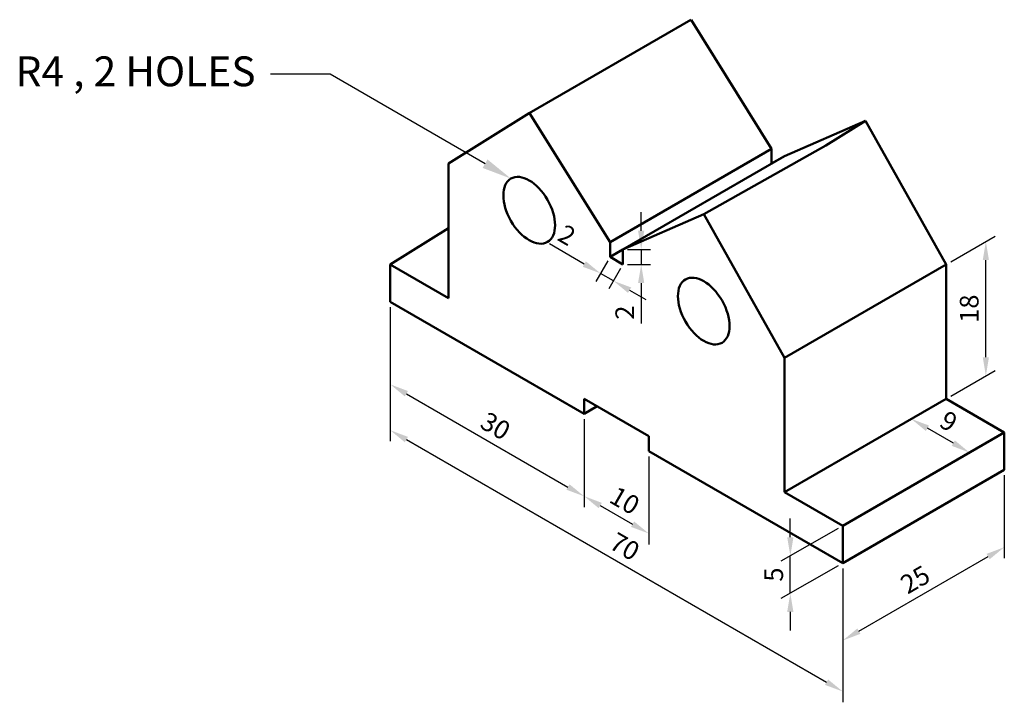
# Model space of a CAD drawing. Units: millimetres. Extents: x 4633 to 4764, y 591 to 682.
import ezdxf
from ezdxf import colors
from ezdxf.entities.mleader import LeaderData, LeaderLine
from ezdxf.math import Vec2, Vec3

# ---------------------------------------------------------------- set-up
doc = ezdxf.new("R2010")
doc.units = ezdxf.units.MM
for name, color, linetype, lineweight in [('M-DIMS', 2, 'Continuous', 25), ('M-OUTL', 7, 'Continuous', 50), ('M-TEXT', 3, 'Continuous', 25)]:
    doc.layers.add(name, color=color, linetype=linetype, lineweight=lineweight)
doc.styles.get("Standard").update_dxf_attribs({"font": 'arial.ttf'})
doc.dimstyles.new('ISO-25', dxfattribs={"dimtxt": 2.5, "dimasz": 2.5, "dimexe": 1.25, "dimexo": 0.625, "dimtad": 1, "dimtxsty": 'Standard', "dimcen": 2.5, "dimadec": 0, "dimazin": 0, "dimtfac": 1, "dimtmove": 0, "dimatfit": 3, "dimfxl": 1, "dimarcsym": 0})

# ---------------------------------------------------------------- blocks, each defined once
blk = doc.blocks.new('*D1')
at = {"layer": 'Defpoints', "color": 0, "transparency": 16777216}
for p in [(4682.17, 644.63), (4708.15, 629.63), (4708.15, 618.56)]:
    blk.add_point(p, dxfattribs=at)
at = {"layer": 'M-DIMS', "color": 0, "lineweight": -2, "transparency": 16777216}
for p, q in [((4682.17, 643.91), (4682.17, 632.12)), ((4684.33, 632.31), (4705.98, 619.81)), ((4708.15, 628.91), (4708.15, 617.12))]:
    blk.add_line(p, q, dxfattribs=at)
at = {"layer": 'M-DIMS', "color": 0, "transparency": 16777216}
for points in [[(4684.54, 632.67), (4684.12, 631.95), (4682.17, 633.56)], [(4706.19, 620.17), (4705.77, 619.45), (4708.15, 618.56)]]:
    blk.add_solid(points, dxfattribs=at)
at = {"layer": 'M-DIMS', "color": 0, "transparency": 16777216, "insert": (4696.11, 627.71), "char_height": 2.5, "attachment_point": 5, "rotation": 330}
blk.add_mtext('30', dxfattribs=at)
blk = doc.blocks.new('*D2')
at = {"layer": 'Defpoints', "color": 0, "transparency": 16777216}
for p in [(4708.15, 629.63), (4716.81, 624.63), (4716.81, 613.58)]:
    blk.add_point(p, dxfattribs=at)
at = {"layer": 'M-DIMS', "color": 0, "lineweight": -2, "transparency": 16777216}
for p, q in [((4708.15, 628.91), (4708.15, 617.13)), ((4716.81, 623.91), (4716.81, 612.13)), ((4710.31, 617.33), (4714.64, 614.83))]:
    blk.add_line(p, q, dxfattribs=at)
at = {"layer": 'M-DIMS', "color": 0, "transparency": 16777216}
for points in [[(4710.52, 617.69), (4710.1, 616.97), (4708.15, 618.58)], [(4714.85, 615.19), (4714.43, 614.47), (4716.81, 613.58)]]:
    blk.add_solid(points, dxfattribs=at)
at = {"layer": 'M-DIMS', "color": 0, "transparency": 16777216, "insert": (4713.43, 617.72), "char_height": 2.5, "attachment_point": 5, "rotation": 330}
blk.add_mtext('10', dxfattribs=at)
blk = doc.blocks.new('*D3')
at = {"layer": 'Defpoints', "color": 0, "transparency": 16777216}
for p in [(4682.17, 644.63), (4742.79, 609.63), (4742.79, 592.42)]:
    blk.add_point(p, dxfattribs=at)
at = {"layer": 'M-DIMS', "color": 0, "lineweight": -2, "transparency": 16777216}
for p, q in [((4682.17, 643.91), (4682.17, 625.97)), ((4684.33, 626.17), (4740.62, 593.67)), ((4742.79, 608.91), (4742.79, 590.97))]:
    blk.add_line(p, q, dxfattribs=at)
at = {"layer": 'M-DIMS', "color": 0, "transparency": 16777216}
for points in [[(4684.54, 626.53), (4684.12, 625.8), (4682.17, 627.42)], [(4740.83, 594.03), (4740.42, 593.3), (4742.79, 592.42)]]:
    blk.add_solid(points, dxfattribs=at)
at = {"layer": 'M-DIMS', "color": 0, "transparency": 16777216, "insert": (4713.43, 611.56), "char_height": 2.5, "attachment_point": 5, "rotation": 330}
blk.add_mtext('70', dxfattribs=at)
blk = doc.blocks.new('*D4')
at = {"layer": 'Defpoints', "color": 0, "transparency": 16777216}
for p in [(4742.79, 614.63), (4735.77, 610.58), (4742.79, 609.63)]:
    blk.add_point(p, dxfattribs=at)
at = {"layer": 'M-DIMS', "color": 0, "lineweight": -2, "transparency": 16777216}
for p, q in [((4735.77, 613.08), (4735.77, 615.58)), ((4742.16, 614.27), (4734.52, 609.86)), ((4735.77, 605.58), (4735.77, 610.58)), ((4742.16, 609.27), (4734.52, 604.86)), ((4735.77, 603.08), (4735.77, 600.58))]:
    blk.add_line(p, q, dxfattribs=at)
at = {"layer": 'M-DIMS', "color": 0, "transparency": 16777216}
for points in [[(4735.35, 613.08), (4736.19, 613.08), (4735.77, 610.58)], [(4735.35, 603.08), (4736.19, 603.08), (4735.77, 605.58)]]:
    blk.add_solid(points, dxfattribs=at)
at = {"layer": 'M-DIMS', "color": 0, "transparency": 16777216, "insert": (4733.87, 608.08), "char_height": 2.5, "attachment_point": 5, "rotation": 90}
blk.add_mtext('5', dxfattribs=at)
blk = doc.blocks.new('*D5')
at = {"layer": 'Defpoints', "color": 0, "transparency": 16777216}
for p in [(4764.44, 622.13), (4764.44, 611.75), (4742.79, 609.63)]:
    blk.add_point(p, dxfattribs=at)
at = {"layer": 'M-DIMS', "color": 0, "lineweight": -2, "transparency": 16777216}
for p, q in [((4764.44, 621.41), (4764.44, 610.3)), ((4744.95, 600.5), (4762.27, 610.5)), ((4742.79, 608.91), (4742.79, 597.8))]:
    blk.add_line(p, q, dxfattribs=at)
at = {"layer": 'M-DIMS', "color": 0, "transparency": 16777216}
for points in [[(4762.07, 610.86), (4762.48, 610.14), (4764.44, 611.75)], [(4744.75, 600.86), (4745.16, 600.14), (4742.79, 599.25)]]:
    blk.add_solid(points, dxfattribs=at)
at = {"layer": 'M-DIMS', "color": 0, "transparency": 16777216, "insert": (4752.66, 607.14), "char_height": 2.5, "attachment_point": 5, "rotation": 30}
blk.add_mtext('25', dxfattribs=at)
blk = doc.blocks.new('*D6')
at = {"layer": 'Defpoints', "color": 0, "transparency": 16777216}
for p in [(4761.97, 652.7), (4756.65, 649.63), (4756.65, 631.63)]:
    blk.add_point(p, dxfattribs=at)
at = {"layer": 'M-DIMS', "color": 0, "lineweight": -2, "transparency": 16777216}
for p, q in [((4757.27, 649.99), (4763.22, 653.42)), ((4761.97, 637.2), (4761.97, 650.2)), ((4757.27, 631.99), (4763.22, 635.42))]:
    blk.add_line(p, q, dxfattribs=at)
at = {"layer": 'M-DIMS', "color": 0, "transparency": 16777216}
for points in [[(4761.55, 650.2), (4762.38, 650.2), (4761.97, 652.7)], [(4761.55, 637.2), (4762.38, 637.2), (4761.97, 634.7)]]:
    blk.add_solid(points, dxfattribs=at)
at = {"layer": 'M-DIMS', "color": 0, "transparency": 16777216, "insert": (4760.06, 643.7), "char_height": 2.5, "attachment_point": 5, "rotation": 90}
blk.add_mtext('18', dxfattribs=at)
blk = doc.blocks.new('*D7')
at = {"layer": 'Defpoints', "color": 0, "transparency": 16777216}
for p in [(4756.65, 631.63), (4751.98, 628.93), (4764.44, 627.13)]:
    blk.add_point(p, dxfattribs=at)
at = {"layer": 'M-DIMS', "color": 0, "lineweight": -2, "transparency": 16777216}
for p, q in [((4756.02, 631.27), (4750.73, 628.21)), ((4757.61, 625.68), (4754.14, 627.68)), ((4763.81, 626.77), (4758.52, 623.71))]:
    blk.add_line(p, q, dxfattribs=at)
at = {"layer": 'M-DIMS', "color": 0, "transparency": 16777216}
for points in [[(4754.35, 628.05), (4753.93, 627.32), (4751.98, 628.93)], [(4757.82, 626.05), (4757.4, 625.32), (4759.77, 624.43)]]:
    blk.add_solid(points, dxfattribs=at)
at = {"layer": 'M-DIMS', "color": 0, "transparency": 16777216, "insert": (4756.83, 628.33), "char_height": 2.5, "attachment_point": 5, "rotation": 330}
blk.add_mtext('9', dxfattribs=at)
blk = doc.blocks.new('*D8')
at = {"layer": 'Defpoints', "color": 0, "transparency": 16777216}
for p in [(4713.34, 651.63), (4713.34, 649.63), (4715.79, 649.63)]:
    blk.add_point(p, dxfattribs=at)
at = {"layer": 'M-DIMS', "color": 0, "lineweight": -2, "transparency": 16777216}
for p, q in [((4715.79, 654.13), (4715.79, 656.63)), ((4713.97, 651.63), (4717.04, 651.63)), ((4715.79, 651.63), (4715.79, 649.63)), ((4713.97, 649.63), (4717.04, 649.63)), ((4715.79, 647.13), (4715.79, 641.72))]:
    blk.add_line(p, q, dxfattribs=at)
at = {"layer": 'M-DIMS', "color": 0, "transparency": 16777216}
for points in [[(4715.37, 654.13), (4716.2, 654.13), (4715.79, 651.63)], [(4715.37, 647.13), (4716.2, 647.13), (4715.79, 649.63)]]:
    blk.add_solid(points, dxfattribs=at)
at = {"layer": 'M-DIMS', "color": 0, "transparency": 16777216, "insert": (4713.91, 643.18), "char_height": 2.5, "attachment_point": 5, "rotation": 90}
blk.add_mtext('2', dxfattribs=at)
blk = doc.blocks.new('*D9')
at = {"layer": 'Defpoints', "color": 0, "transparency": 16777216}
for p in [(4711.61, 650.63), (4713.34, 649.63), (4710.34, 648.43)]:
    blk.add_point(p, dxfattribs=at)
at = {"layer": 'M-DIMS', "color": 0, "lineweight": -2, "transparency": 16777216}
for p, q in [((4708.17, 649.68), (4703.49, 652.38)), ((4711.3, 650.09), (4709.71, 647.34)), ((4713.03, 649.09), (4711.45, 646.34)), ((4712.07, 647.43), (4710.34, 648.43)), ((4714.24, 646.18), (4716.4, 644.93))]:
    blk.add_line(p, q, dxfattribs=at)
at = {"layer": 'M-DIMS', "color": 0, "transparency": 16777216}
for points in [[(4708.38, 650.04), (4707.97, 649.31), (4710.34, 648.43)], [(4714.45, 646.54), (4714.03, 645.81), (4712.07, 647.43)]]:
    blk.add_solid(points, dxfattribs=at)
at = {"layer": 'M-DIMS', "color": 0, "transparency": 16777216, "insert": (4705.69, 653.28), "char_height": 2.5, "attachment_point": 5, "rotation": 330}
blk.add_mtext('2', dxfattribs=at)

msp = doc.modelspace()

# ---------------------------------------------------------------- linework, layer by layer
at = {"layer": 'M-OUTL'}
for p, q in [((4722.437, 682.379), (4700.787, 669.879)), ((4733.263, 665.129), (4722.487, 682.41)), ((4689.961, 663.129), (4700.787, 669.879)), ((4711.612, 652.629), (4700.837, 669.91)), ((4734.995, 664.129), (4745.82, 668.879)), ((4740.513, 665.57), (4745.82, 668.879)), ((4756.645, 649.629), (4745.82, 668.879)), ((4733.263, 665.129), (4711.612, 652.629)), ((4724.169, 656.379), (4740.513, 665.57)), ((4733.263, 663.129), (4733.263, 665.129)), ((4713.344, 651.629), (4734.995, 664.129)), ((4734.995, 664.129), (4733.263, 663.129)), ((4689.961, 645.129), (4689.961, 663.129)), ((4713.344, 651.629), (4724.169, 656.379)), ((4734.995, 637.129), (4724.169, 656.379)), ((4682.167, 649.629), (4689.961, 654.489)), ((4711.612, 650.629), (4711.612, 652.629)), ((4711.612, 650.629), (4713.344, 651.629)), ((4711.612, 650.629), (4713.344, 649.629)), ((4713.344, 649.629), (4711.612, 650.629)), ((4713.344, 649.629), (4713.344, 651.629)), ((4682.167, 644.629), (4682.167, 649.629)), ((4682.167, 649.629), (4689.961, 645.129)), ((4734.995, 637.129), (4756.645, 649.629)), ((4756.645, 631.629), (4756.645, 649.629)), ((4682.167, 644.629), (4708.148, 629.629)), ((4734.995, 619.129), (4734.995, 637.129)), ((4708.148, 629.629), (4708.148, 631.629)), ((4708.148, 631.629), (4716.808, 626.629)), ((4708.148, 629.629), (4709.88, 630.629)), ((4734.995, 619.129), (4756.645, 631.629)), ((4764.44, 627.129), (4756.645, 631.629)), ((4716.808, 626.629), (4716.808, 624.629)), ((4742.789, 614.629), (4764.44, 627.129)), ((4764.44, 622.129), (4764.44, 627.129)), ((4716.808, 624.629), (4742.789, 609.629)), ((4742.789, 609.629), (4764.44, 622.129)), ((4742.789, 614.629), (4734.995, 619.129)), ((4742.789, 609.629), (4742.789, 614.629))]:
    msp.add_line(p, q, dxfattribs=at)
for centre in [(4700.787, 656.879), (4724.169, 643.379)]:
    msp.add_ellipse(centre, major_axis=(2.449, -4.243), ratio=0.5773503, dxfattribs=at)

# ---------------------------------------------------------------- dimensions: what is measured, and where the dimension line sits
at = {"layer": 'M-DIMS'}
for p1, p2, distance, picture, middle in [((4713.344, 651.629), (4713.344, 649.629), 2.444, '*D8', (4713.908, 643.176)), ((4713.344, 649.629), (4711.612, 650.629), 2.544, '*D9', (4705.691, 653.28)), ((4756.645, 631.629), (4756.645, 649.629), -5.32, '*D6', (4760.064, 643.701)), ((4682.167, 644.629), (4708.148, 629.629), -9.584, '*D1', (4696.109, 627.71)), ((4682.167, 644.629), (4742.789, 609.629), -14.907, '*D3', (4713.429, 611.562)), ((4764.44, 627.129), (4756.645, 631.629), 4.667, '*D7', (4756.826, 628.331)), ((4708.148, 629.629), (4716.808, 624.629), -9.571, '*D2', (4713.429, 617.724)), ((4742.789, 609.629), (4764.44, 622.129), -8.99, '*D5', (4752.664, 607.145)), ((4742.789, 609.629), (4742.789, 614.629), 7.018, '*D4', (4733.874, 608.077))]:
    dim = msp.add_aligned_dim(p1=p1, p2=p2, distance=distance, dimstyle='ISO-25', override={"dimclrd": 0, "dimclre": 0, "dimclrt": 0}, dxfattribs=at)
    dim.commit()
    dim.dimension.update_dxf_attribs({"geometry": picture, "text_midpoint": middle})

# ---------------------------------------------------------------- leaders
at = {"layer": 'M-TEXT'}
ml = msp.add_multileader_mtext('Standard', dxfattribs=at)
ml.set_content('R4 , 2 HOLES ', color=256)
ml.set_leader_properties()
ml.build(insert=Vec2(0, 0))
ctx = ml.context
ctx.base_point, ctx.plane_origin = Vec3(4627.453, 675.099), Vec3(4698.337, 661.122)
ctx.text_align_type = 2
notes = []
notes.append((ctx, [(0, (1, 1, 0), (4674.127, 675.099), (-1, 0), 8, [(0, [(4698.337, 661.122)], 0, [])])]))
ctx.mtext.insert, ctx.mtext.alignment, ctx.mtext.flow_direction = Vec3(4664.127, 677.495), 3, 5
for ctx, leaders in notes:
    for number, flags, end, landing, length, lines in leaders:
        leader = LeaderData()
        leader.index, (leader.has_last_leader_line, leader.has_dogleg_vector, leader.attachment_direction) = number, flags
        leader.last_leader_point, leader.dogleg_vector, leader.dogleg_length = Vec3(end), Vec3(landing), length
        for number, points, colour, breaks in lines:
            line = LeaderLine()
            line.index, line.vertices, line.color, line.breaks = number, Vec3.list(points), colors.encode_raw_color(colour), breaks
            leader.lines.append(line)
        ctx.leaders.append(leader)

doc.saveas('drawing.dxf')
